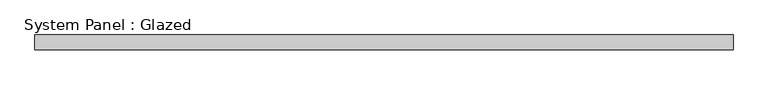
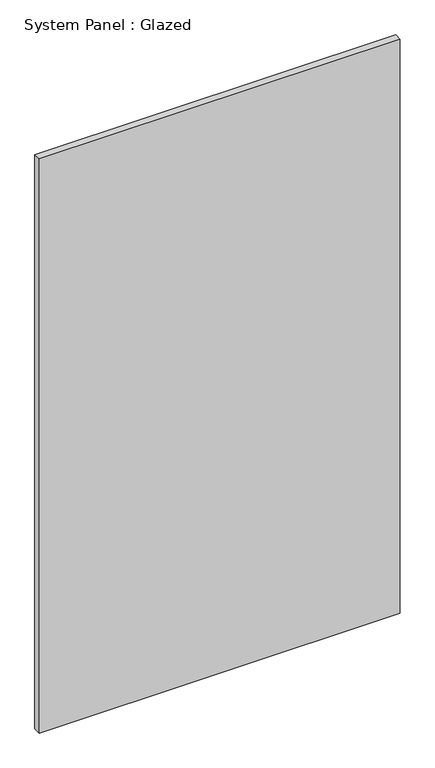
"""IFC4 building model written with IfcOpenShell, lengths in millimetres: plate geometry, System Panel : Glazed."""

from ifc_helpers import new_model, si_unit, origin, origin_with_axes, place, context, project, spatial, polyline, outline, extrude, source, transform, mapped, element, save


def system_panel_glazed_6a2d4635(model_context):
    return source(origin(), model_context, "Body", "SweptSolid", [
        extrude(outline(polyline([(596.9, -44.45), (-596.9, -44.45), (-596.9, -19.05), (596.9, -19.05), (596.9, -44.45)])), origin_with_axes(), (0.0, 0.0, 1.0), 2006.6),
    ])


if __name__ == "__main__":
    model = new_model("IFC4")
    model_context = context("Model", 3, world=origin())
    ifc_project = project(units=[si_unit("LENGTHUNIT", "METRE", prefix="MILLI")], contexts=[model_context])
    site = spatial("IfcSite", under=ifc_project)
    building = spatial("IfcBuilding", under=site)
    placement = place(None, origin())
    system_panel_glazed_shape = system_panel_glazed_6a2d4635(model_context)
    element("IfcPlate", 1, ObjectType="System Panel : Glazed", at=placement, inside=building, context=model_context, shape_type="MappedRepresentation", body=[
        mapped(system_panel_glazed_shape, transform((0.0, 0.0, 0.0), x_axis=(1.0, 0.0, 0.0), y_axis=(0.0, 1.0, 0.0), z_axis=(0.0, 0.0, 1.0))),
    ])
    save(model, "model.ifc")

# Revit data of these elements
# Type "System Panel : Glazed"
#   Construction Type Id = "GSP4R"
#   Analytic Construction = "1/8 in Pilkington single glazing"
#   Visual Light Transmittance = 0.9
#   Solar Heat Gain Coefficient = 0.86
#   Heat Transfer Coefficient (U) = 1.18115 BTU/(h·ft²·°F)
#   Define Thermal Properties by = 1
# Element 1 (IfcPlate, "System Panel : Glazed")
#   Materials on its faces: "Glass"
# Materials
#   "Glass": class "Glass", colour RGB 0 128 192, transparency 0.75, Description = "Soda Lime Glass", Cost = 0
